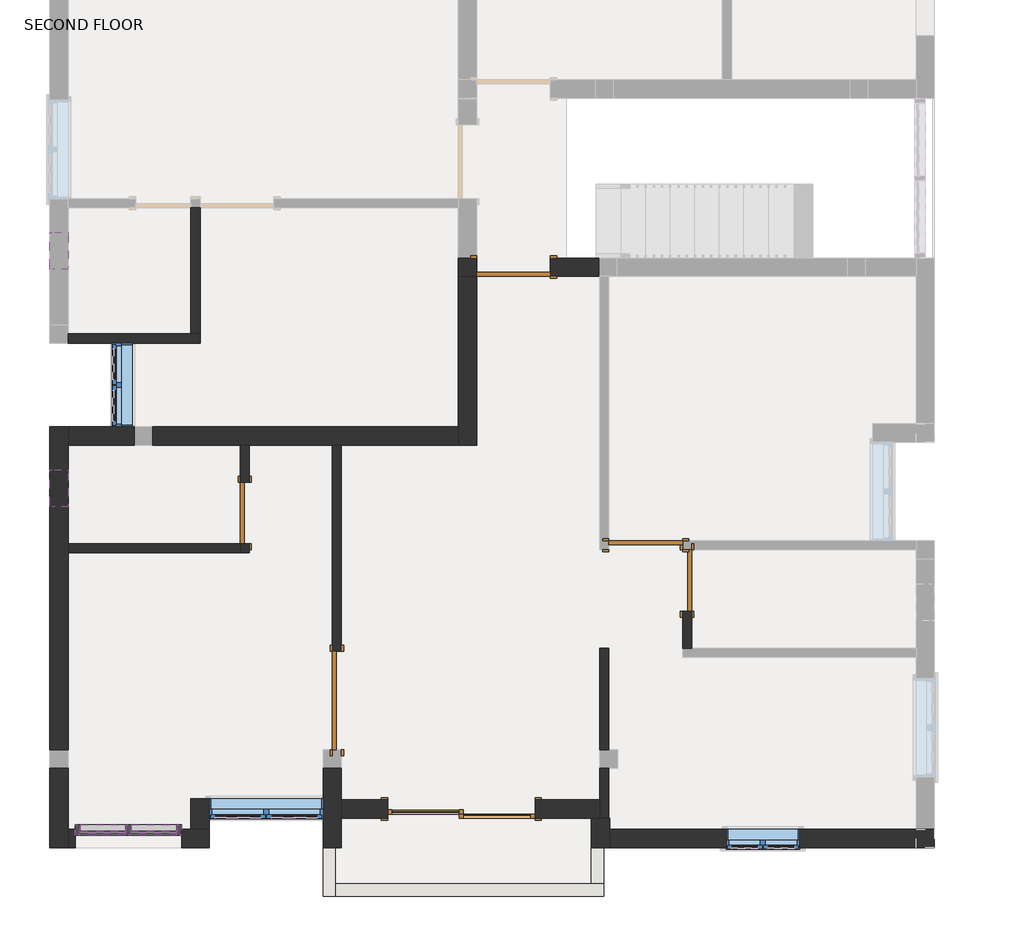
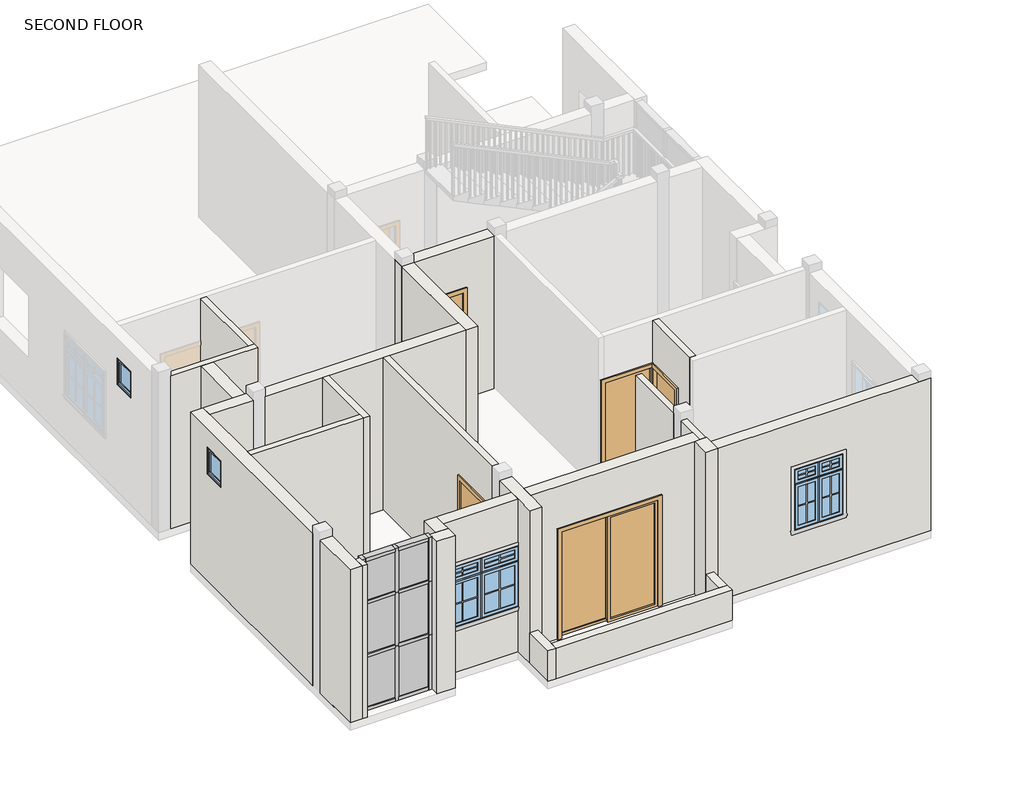
# One storey, part 1 of 6: 25 walls, 17 members, 6 doors, 6 plates, 5 windows.
"""IFC4 building model written with IfcOpenShell, lengths in millimetres."""

from ifc_helpers import new_model, si_unit, frame, origin, place, context, project, spatial, polyline, outline, extrude, faceted_brep, transform, mapped, element, save
from components import door_d4d75d1e, door_78caadf7, single_flush_3_x7_0ca8825f, single_flush_3_x7_305aa2a5, single_flush_4_x7_9343de66, member_6f432376, member_6103f85b, member_e80433b6, member_a715cb85, member_69c8e218, member_c4de40ee, member_049a2e78, member_5cd4c5ac, system_panel_glazed_fbef02e7, system_panel_glazed_b4a8312c, window_abb441dd, window_35f3c129, window_casement_double_awning_double_3_x4_7dc4ce09, window_c5cb33f6

model = new_model("IFC4")

# Units and contexts
model_context = context("Model", 3, world=origin())
ifc_project = project(units=[si_unit("LENGTHUNIT", "METRE", prefix="MILLI")], contexts=[model_context])

# Site, building, storey
site = spatial("IfcSite", under=ifc_project)
building = spatial("IfcBuilding", under=site)
storey = spatial("IfcBuildingStorey", under=building, Name="SECOND FLOOR", Elevation=6400.8)

# Doors
placement = place(None, origin())
door_shape = door_d4d75d1e(model_context)
element("IfcDoor", 1, ObjectType="Door-Double-Sliding : 72\" x 84\"", at=placement, inside=storey, context=model_context, shape_type="MappedRepresentation", body=[
    mapped(door_shape, transform((-1663.0865981, -7209.8212413, 6400.8), x_axis=(-1.0, 0.0, 0.0), y_axis=(0.0, -1.0, 0.0), z_axis=(0.0, 0.0, 1.0))),
])
door_2_shape = door_78caadf7(model_context)
element("IfcDoor", 2, ObjectType="Single-Flush : 2'6\"X7'", at=placement, inside=storey, context=model_context, shape_type="MappedRepresentation", body=[
    mapped(door_2_shape, transform((-4349.1365981, -3666.5212413, 6400.8), x_axis=(0.0, -1.0, 0.0), y_axis=(1.0, 0.0, 0.0), z_axis=(0.0, 0.0, 1.0))),
])
element("IfcDoor", 3, ObjectType="Single-Flush : 2'6\"X7'", at=placement, inside=storey, context=model_context, shape_type="MappedRepresentation", body=[
    mapped(door_2_shape, transform((1137.2634019, -4504.7212413, 6400.8), x_axis=(0.0, 1.0, 0.0), y_axis=(-1.0, 0.0, 0.0), z_axis=(0.0, 0.0, 1.0))),
])
single_flush_3_x7_shape = single_flush_3_x7_0ca8825f(model_context)
element("IfcDoor", 4, ObjectType="Single-Flush : 3'X7'", at=placement, inside=storey, context=model_context, shape_type="MappedRepresentation", body=[
    mapped(single_flush_3_x7_shape, transform((-1015.3865981, -618.5212413, 6400.8), x_axis=(-1.0, 0.0, 0.0), y_axis=(0.0, -1.0, 0.0), z_axis=(0.0, 0.0, 1.0))),
])
single_flush_3_x7_2_shape = single_flush_3_x7_305aa2a5(model_context)
element("IfcDoor", 5, ObjectType="Single-Flush : 3'X7'", at=placement, inside=storey, context=model_context, shape_type="MappedRepresentation", body=[
    mapped(single_flush_3_x7_2_shape, transform((622.9134019, -4066.5712413, 6400.8), x_axis=(-1.0, 0.0, 0.0), y_axis=(0.0, -1.0, 0.0), z_axis=(0.0, 0.0, 1.0))),
])
single_flush_4_x7_shape = single_flush_4_x7_9343de66(model_context)
element("IfcDoor", 6, ObjectType="Single-Flush : 4'X7'", at=placement, inside=storey, context=model_context, shape_type="MappedRepresentation", body=[
    mapped(single_flush_4_x7_shape, transform((-3206.1365981, -5990.6212413, 6400.8), x_axis=(0.0, -1.0, 0.0), y_axis=(1.0, 0.0, 0.0), z_axis=(0.0, 0.0, 1.0))),
])

# Members
member_shape = member_6f432376(model_context)
element("IfcMember", 7, ObjectType="Rectangular Mullion : 2.5\" x 5\" rectangular", at=placement, inside=storey, context=model_context, shape_type="MappedRepresentation", body=[
    mapped(member_shape, transform((-5193.6865981, -7597.1712413, 9448.8), x_axis=(0.0, 0.0, 1.0), y_axis=(0.0, -1.0, 0.0), z_axis=(1.0, 0.0, 0.0))),
])
element("IfcMember", 8, ObjectType="Rectangular Mullion : 2.5\" x 5\" rectangular", at=placement, inside=storey, context=model_context, shape_type="MappedRepresentation", body=[
    mapped(member_shape, transform((-5822.3365981, -7597.1712413, 9448.8), x_axis=(0.0, 0.0, 1.0), y_axis=(0.0, -1.0, 0.0), z_axis=(1.0, 0.0, 0.0))),
])
element("IfcMember", 9, ObjectType="Rectangular Mullion : 2.5\" x 5\" rectangular", at=placement, inside=storey, context=model_context, shape_type="MappedRepresentation", body=[
    mapped(member_shape, transform((-6387.4865981, -7597.1712413, 6400.8), x_axis=(0.0, 0.0, -1.0), y_axis=(0.0, -1.0, 0.0), z_axis=(-1.0, 0.0, 0.0))),
])
element("IfcMember", 10, ObjectType="Rectangular Mullion : 2.5\" x 5\" rectangular", at=placement, inside=storey, context=model_context, shape_type="MappedRepresentation", body=[
    mapped(member_shape, transform((-5758.8365981, -7597.1712413, 6400.8), x_axis=(0.0, 0.0, -1.0), y_axis=(0.0, -1.0, 0.0), z_axis=(-1.0, 0.0, 0.0))),
])
member_2_shape = member_6103f85b(model_context)
element("IfcMember", 11, ObjectType="Rectangular Mullion : 2.5\" x 5\" rectangular", at=placement, inside=storey, context=model_context, shape_type="MappedRepresentation", body=[
    mapped(member_2_shape, transform((-5822.3365981, -7597.1712413, 7499.35), x_axis=(0.0, 0.0, 1.0), y_axis=(0.0, -1.0, 0.0), z_axis=(1.0, 0.0, 0.0))),
])
element("IfcMember", 12, ObjectType="Rectangular Mullion : 2.5\" x 5\" rectangular", at=placement, inside=storey, context=model_context, shape_type="MappedRepresentation", body=[
    mapped(member_2_shape, transform((-5822.3365981, -7597.1712413, 8566.15), x_axis=(0.0, 0.0, 1.0), y_axis=(0.0, -1.0, 0.0), z_axis=(1.0, 0.0, 0.0))),
])
element("IfcMember", 13, ObjectType="Rectangular Mullion : 2.5\" x 5\" rectangular", at=placement, inside=storey, context=model_context, shape_type="MappedRepresentation", body=[
    mapped(member_2_shape, transform((-5193.6865981, -7597.1712413, 7499.35), x_axis=(0.0, 0.0, 1.0), y_axis=(0.0, -1.0, 0.0), z_axis=(1.0, 0.0, 0.0))),
])
element("IfcMember", 14, ObjectType="Rectangular Mullion : 2.5\" x 5\" rectangular", at=placement, inside=storey, context=model_context, shape_type="MappedRepresentation", body=[
    mapped(member_2_shape, transform((-5193.6865981, -7597.1712413, 8566.15), x_axis=(0.0, 0.0, 1.0), y_axis=(0.0, -1.0, 0.0), z_axis=(1.0, 0.0, 0.0))),
])
member_3_shape = member_e80433b6(model_context)
element("IfcMember", 15, ObjectType="Rectangular Mullion : 2.5\" x 5\" rectangular", at=placement, inside=storey, context=model_context, shape_type="MappedRepresentation", body=[
    mapped(member_3_shape, transform((-5790.5865981, -7597.1712413, 6400.8), x_axis=(1.0, 0.0, 0.0), y_axis=(0.0, -1.0, 0.0), z_axis=(0.0, 0.0, -1.0))),
])
member_4_shape = member_a715cb85(model_context)
element("IfcMember", 16, ObjectType="Rectangular Mullion : 2.5\" x 5\" rectangular", at=placement, inside=storey, context=model_context, shape_type="MappedRepresentation", body=[
    mapped(member_4_shape, transform((-5790.5865981, -7597.1712413, 7499.35), x_axis=(1.0, 0.0, 0.0), y_axis=(0.0, -1.0, 0.0), z_axis=(0.0, 0.0, -1.0))),
])
member_5_shape = member_69c8e218(model_context)
element("IfcMember", 17, ObjectType="Rectangular Mullion : 2.5\" x 5\" rectangular", at=placement, inside=storey, context=model_context, shape_type="MappedRepresentation", body=[
    mapped(member_5_shape, transform((-5130.1865981, -7597.1712413, 6400.8), x_axis=(1.0, 0.0, 0.0), y_axis=(0.0, -1.0, 0.0), z_axis=(0.0, 0.0, -1.0))),
])
member_6_shape = member_c4de40ee(model_context)
element("IfcMember", 18, ObjectType="Rectangular Mullion : 2.5\" x 5\" rectangular", at=placement, inside=storey, context=model_context, shape_type="MappedRepresentation", body=[
    mapped(member_6_shape, transform((-5130.1865981, -7597.1712413, 7499.35), x_axis=(1.0, 0.0, 0.0), y_axis=(0.0, -1.0, 0.0), z_axis=(0.0, 0.0, -1.0))),
])
element("IfcMember", 19, ObjectType="Rectangular Mullion : 2.5\" x 5\" rectangular", at=placement, inside=storey, context=model_context, shape_type="MappedRepresentation", body=[
    mapped(member_5_shape, transform((-6450.9865981, -7597.1712413, 7499.35), x_axis=(-1.0, 0.0, 0.0), y_axis=(0.0, -1.0, 0.0), z_axis=(0.0, 0.0, 1.0))),
])
element("IfcMember", 20, ObjectType="Rectangular Mullion : 2.5\" x 5\" rectangular", at=placement, inside=storey, context=model_context, shape_type="MappedRepresentation", body=[
    mapped(member_6_shape, transform((-6450.9865981, -7597.1712413, 8566.15), x_axis=(-1.0, 0.0, 0.0), y_axis=(0.0, -1.0, 0.0), z_axis=(0.0, 0.0, 1.0))),
])
member_7_shape = member_049a2e78(model_context)
element("IfcMember", 21, ObjectType="Rectangular Mullion : 2.5\" x 5\" rectangular", at=placement, inside=storey, context=model_context, shape_type="MappedRepresentation", body=[
    mapped(member_7_shape, transform((-5790.5865981, -7597.1712413, 8566.15), x_axis=(1.0, 0.0, 0.0), y_axis=(0.0, -1.0, 0.0), z_axis=(0.0, 0.0, -1.0))),
])
member_8_shape = member_5cd4c5ac(model_context)
element("IfcMember", 22, ObjectType="Rectangular Mullion : 2.5\" x 5\" rectangular", at=placement, inside=storey, context=model_context, shape_type="MappedRepresentation", body=[
    mapped(member_8_shape, transform((-5130.1865981, -7597.1712413, 8566.15), x_axis=(1.0, 0.0, 0.0), y_axis=(0.0, -1.0, 0.0), z_axis=(0.0, 0.0, -1.0))),
])
element("IfcMember", 23, ObjectType="Rectangular Mullion : 2.5\" x 5\" rectangular", at=placement, inside=storey, context=model_context, shape_type="MappedRepresentation", body=[
    mapped(member_8_shape, transform((-6450.9865981, -7597.1712413, 9448.8), x_axis=(-1.0, 0.0, 0.0), y_axis=(0.0, -1.0, 0.0), z_axis=(0.0, 0.0, 1.0))),
])

# Plates
system_panel_glazed_shape = system_panel_glazed_fbef02e7(model_context)
element("IfcPlate", 24, ObjectType="System Panel : Glazed", at=placement, inside=storey, context=model_context, shape_type="MappedRepresentation", body=[
    mapped(system_panel_glazed_shape, transform((-6104.9115981, -7597.1712413, 6464.3), x_axis=(1.0, 0.0, 0.0), y_axis=(0.0, 1.0, 0.0), z_axis=(0.0, 0.0, 1.0))),
])
element("IfcPlate", 25, ObjectType="System Panel : Glazed", at=placement, inside=storey, context=model_context, shape_type="MappedRepresentation", body=[
    mapped(system_panel_glazed_shape, transform((-6104.9115981, -7597.1712413, 7531.1), x_axis=(1.0, 0.0, 0.0), y_axis=(0.0, 1.0, 0.0), z_axis=(0.0, 0.0, 1.0))),
])
element("IfcPlate", 26, ObjectType="System Panel : Glazed", at=placement, inside=storey, context=model_context, shape_type="MappedRepresentation", body=[
    mapped(system_panel_glazed_shape, transform((-5476.2615981, -7597.1712413, 6464.3), x_axis=(1.0, 0.0, 0.0), y_axis=(0.0, 1.0, 0.0), z_axis=(0.0, 0.0, 1.0))),
])
element("IfcPlate", 27, ObjectType="System Panel : Glazed", at=placement, inside=storey, context=model_context, shape_type="MappedRepresentation", body=[
    mapped(system_panel_glazed_shape, transform((-5476.2615981, -7597.1712413, 7531.1), x_axis=(1.0, 0.0, 0.0), y_axis=(0.0, 1.0, 0.0), z_axis=(0.0, 0.0, 1.0))),
])
system_panel_glazed_2_shape = system_panel_glazed_b4a8312c(model_context)
element("IfcPlate", 28, ObjectType="System Panel : Glazed", at=placement, inside=storey, context=model_context, shape_type="MappedRepresentation", body=[
    mapped(system_panel_glazed_2_shape, transform((-6104.9115981, -7597.1712413, 8597.9), x_axis=(1.0, 0.0, 0.0), y_axis=(0.0, 1.0, 0.0), z_axis=(0.0, 0.0, 1.0))),
])
element("IfcPlate", 29, ObjectType="System Panel : Glazed", at=placement, inside=storey, context=model_context, shape_type="MappedRepresentation", body=[
    mapped(system_panel_glazed_2_shape, transform((-5476.2615981, -7597.1712413, 8597.9), x_axis=(1.0, 0.0, 0.0), y_axis=(0.0, 1.0, 0.0), z_axis=(0.0, 0.0, 1.0))),
])

# Walls
element("IfcWall", 30, ObjectType="4.5\"", at=placement, inside=storey, context=model_context, shape_type="Brep", body=[
    faceted_brep([(-6539.8865981, -1558.3212413, 6400.8), (-5974.2886947, -1558.3212413, 6400.8), (-5745.6886947, -1558.3212413, 6400.8), (-4901.5865981, -1558.3212413, 6400.8), (-4901.5865981, -1558.3212413, 9448.8), (-5745.6886947, -1558.3212413, 9448.8), (-5974.2886947, -1558.3212413, 9448.8), (-6539.8865981, -1558.3212413, 9448.8), (-6539.8865981, -1444.0212413, 6400.8), (-6539.8865981, -1444.0212413, 9448.8), (-5015.8865981, -1444.0212413, 9448.8), (-4901.5865981, -1444.0212413, 9448.8), (-4901.5865981, -1444.0212413, 6400.8), (-5015.8865981, -1444.0212413, 6400.8)], [[[0, 1, 2, 3, 4, 5, 6, 7]], [[8, 9, 10, 11, 12, 13]], [[3, 2, 1, 0, 8, 13, 12]], [[7, 6, 5, 4, 11, 10, 9]], [[0, 7, 9, 8]], [[4, 3, 12, 11]]]),
])
element("IfcWall", 31, ObjectType="4.5\"", at=placement, inside=storey, context=model_context, shape_type="SweptSolid", body=[
    extrude(outline(polyline([(-4901.5865981, 118.0787587), (-4901.5865981, -1444.0212413), (-5015.8865981, -1444.0212413), (-5015.8865981, 118.0787587), (-4901.5865981, 118.0787587)])), frame((0.0, 0.0, 6400.8), z_axis=(0.0, 0.0, 1.0), x_axis=(1.0, 0.0, 0.0)), (0.0, 0.0, 1.0), 3048.0),
])
element("IfcWall", 32, ObjectType="4.5\"", at=placement, inside=storey, context=model_context, shape_type="Brep", body=[
    faceted_brep([(-4406.2865981, -4047.5212413, 8534.4), (-4406.2865981, -4047.5212413, 6400.8), (-4406.2865981, -4161.8212413, 6400.8), (-4406.2865981, -4161.8212413, 9448.8), (-4406.2865981, -4047.5212413, 9448.8), (-4406.2865981, -2828.3212413, 9448.8), (-4406.2865981, -2828.3212413, 6400.8), (-4406.2865981, -3285.5212413, 6400.8), (-4406.2865981, -3285.5212413, 8534.4), (-4291.9865981, -4161.8212413, 6400.8), (-4291.9865981, -4047.5212413, 6400.8), (-4291.9865981, -4047.5212413, 8534.4), (-4291.9865981, -3285.5212413, 8534.4), (-4291.9865981, -3285.5212413, 6400.8), (-4291.9865981, -2828.3212413, 6400.8), (-4291.9865981, -2828.3212413, 9448.8), (-4291.9865981, -4161.8212413, 9448.8)], [[[0, 1, 2, 3, 4, 5, 6, 7, 8]], [[9, 10, 11, 12, 13, 14, 15, 16]], [[7, 6, 14, 13]], [[2, 1, 10, 9]], [[5, 4, 3, 16, 15]], [[6, 5, 15, 14]], [[3, 2, 9, 16]], [[11, 10, 1, 0]], [[12, 11, 0, 8]], [[13, 12, 8, 7]]]),
])
element("IfcWall", 33, ObjectType="4.5\"", at=placement, inside=storey, context=model_context, shape_type="SweptSolid", body=[
    extrude(outline(polyline([(-6539.8865981, -4047.5212413), (-4406.2865981, -4047.5212413), (-4406.2865981, -4161.8212413), (-6539.8865981, -4161.8212413), (-6539.8865981, -4047.5212413)])), frame((0.0, 0.0, 6400.8), z_axis=(0.0, 0.0, 1.0), x_axis=(1.0, 0.0, 0.0)), (0.0, 0.0, 1.0), 3048.0),
])
element("IfcWall", 34, ObjectType="4.5\"", at=placement, inside=storey, context=model_context, shape_type="SweptSolid", body=[
    extrude(outline(polyline([(-6600.2212413, 9448.8), (-2828.3212413, 9448.8), (-2828.3212413, 6400.8), (-5381.0212413, 6400.8), (-5381.0212413, 8534.4), (-6600.2212413, 8534.4), (-6600.2212413, 9448.8)])), frame((-3263.2865981, 0.0, 0.0), z_axis=(1.0, 0.0, 0.0), x_axis=(0.0, 1.0, 0.0)), (0.0, 0.0, 1.0), 114.3),
])
element("IfcWall", 35, ObjectType="4.5\"", at=placement, inside=storey, context=model_context, shape_type="SweptSolid", body=[
    extrude(outline(polyline([(-5342.9212413, 9448.8), (-4123.7212413, 9448.8), (-4123.7212413, 8534.4), (-4885.7212413, 8534.4), (-4885.7212413, 6400.8), (-5342.9212413, 6400.8), (-5342.9212413, 9448.8)])), frame((1080.1134019, 0.0, 0.0), z_axis=(1.0, 0.0, 0.0), x_axis=(0.0, 1.0, 0.0)), (0.0, 0.0, 1.0), 114.3),
])
element("IfcWall", 36, ObjectType="4.5\"", at=placement, inside=storey, context=model_context, shape_type="SweptSolid", body=[
    extrude(outline(polyline([(51.4134019, -6601.1424416), (51.4134019, -5342.9212413), (165.7134019, -5342.9212413), (165.7134019, -6601.1424416), (51.4134019, -6601.1424416)])), frame((0.0, 0.0, 6400.8), z_axis=(0.0, 0.0, 1.0), x_axis=(1.0, 0.0, 0.0)), (0.0, 0.0, 1.0), 3048.0),
])
element("IfcWall", 37, ObjectType="4.5\"", at=placement, inside=storey, context=model_context, shape_type="Brep", body=[
    faceted_brep([(51.4134019, -6829.7424416, 6400.8), (51.4134019, -7222.5212413, 6400.8), (51.4134019, -7451.1212413, 6400.8), (51.4134019, -7451.1212413, 9448.8), (51.4134019, -7222.5212413, 9448.8), (51.4134019, -6829.7424416, 9448.8), (165.7134019, -6829.7424416, 6400.8), (165.7134019, -6829.7424416, 9448.8), (165.7134019, -7451.1212413, 9448.8), (165.7134019, -7451.1212413, 6400.8)], [[[0, 1, 2, 3, 4, 5]], [[6, 7, 8, 9]], [[2, 1, 0, 6, 9]], [[5, 4, 3, 8, 7]], [[0, 5, 7, 6]], [[3, 2, 9, 8]]]),
])
element("IfcWall", 38, ObjectType="6\"", at=placement, inside=storey, context=model_context, shape_type="Brep", body=[
    faceted_brep([(-3377.5865981, -7819.4212413, 6400.8), (-3377.5865981, -8416.3212413, 6400.8), (-3377.5865981, -8416.3212413, 7010.4), (-3377.5865981, -7819.4212413, 7010.4), (-3225.1865981, -7819.4212413, 6400.8), (-3225.1865981, -7819.4212413, 7010.4), (-3225.1865981, -8263.9212413, 7010.4), (-3225.1865981, -8416.3212413, 7010.4), (-3225.1865981, -8416.3212413, 6400.8), (-3225.1865981, -8263.9212413, 6400.8)], [[[0, 1, 2, 3]], [[4, 5, 6, 7, 8, 9]], [[1, 0, 4, 9, 8]], [[3, 2, 7, 6, 5]], [[0, 3, 5, 4]], [[2, 1, 8, 7]]]),
])
element("IfcWall", 39, ObjectType="6\"", at=placement, inside=storey, context=model_context, shape_type="Brep", body=[
    faceted_brep([(-3225.1865981, -8416.3212413, 6400.8), (102.2134019, -8416.3212413, 6400.8), (102.2134019, -8416.3212413, 7010.4), (-3225.1865981, -8416.3212413, 7010.4), (-3225.1865981, -8263.9212413, 6400.8), (-3225.1865981, -8263.9212413, 7010.4), (-50.1865981, -8263.9212413, 7010.4), (102.2134019, -8263.9212413, 7010.4), (102.2134019, -8263.9212413, 6400.8), (-50.1865981, -8263.9212413, 6400.8)], [[[0, 1, 2, 3]], [[4, 5, 6, 7, 8, 9]], [[1, 0, 4, 9, 8]], [[3, 2, 7, 6, 5]], [[0, 3, 5, 4]], [[2, 1, 8, 7]]]),
])
element("IfcWall", 40, ObjectType="6\"", at=placement, inside=storey, context=model_context, shape_type="SweptSolid", body=[
    extrude(outline(polyline([(102.2134019, -7819.4212413), (102.2134019, -8263.9212413), (-50.1865981, -8263.9212413), (-50.1865981, -7819.4212413), (102.2134019, -7819.4212413)])), frame((0.0, 0.0, 6400.8), z_axis=(0.0, 0.0, 1.0), x_axis=(1.0, 0.0, 0.0)), (0.0, 0.0, 1.0), 609.6),
])
element("IfcWall", 41, ObjectType="9\"", at=placement, inside=storey, context=model_context, shape_type="Brep", body=[
    faceted_brep([(-6768.4865981, -2599.7212413, 6400.8), (-6768.4865981, -6601.1424416, 6400.8), (-6768.4865981, -6601.1424416, 9448.8), (-6768.4865981, -2599.7212413, 9448.8), (-6768.4865981, -3133.1212413, 9067.8), (-6768.4865981, -3590.3212413, 9067.8), (-6768.4865981, -3590.3212413, 8534.4), (-6768.4865981, -3133.1212413, 8534.4), (-6539.8865981, -2599.7212413, 6400.8), (-6539.8865981, -2599.7212413, 9448.8), (-6539.8865981, -2828.3212413, 9448.8), (-6539.8865981, -4047.5212413, 9448.8), (-6539.8865981, -4161.8212413, 9448.8), (-6539.8865981, -6601.1424416, 9448.8), (-6539.8865981, -6601.1424416, 6400.8), (-6539.8865981, -4161.8212413, 6400.8), (-6539.8865981, -4047.5212413, 6400.8), (-6539.8865981, -2828.3212413, 6400.8), (-6539.8865981, -3133.1212413, 9067.8), (-6539.8865981, -3133.1212413, 8534.4), (-6539.8865981, -3590.3212413, 8534.4), (-6539.8865981, -3590.3212413, 9067.8)], [[[0, 1, 2, 3], [4, 5, 6, 7]], [[8, 9, 10, 11, 12, 13, 14, 15, 16, 17], [18, 19, 20, 21]], [[1, 0, 8, 17, 16, 15, 14]], [[2, 1, 14, 13]], [[3, 2, 13, 12, 11, 10, 9]], [[0, 3, 9, 8]], [[19, 18, 4, 7]], [[20, 19, 7, 6]], [[21, 20, 6, 5]], [[18, 21, 5, 4]]]),
])
element("IfcWall", 42, ObjectType="9\"", at=placement, inside=storey, context=model_context, shape_type="Brep", body=[
    faceted_brep([(-6768.4865981, -6829.7424416, 6400.8), (-6768.4865981, -7819.4212413, 6400.8), (-6768.4865981, -7819.4212413, 9448.8), (-6768.4865981, -6829.7424416, 9448.8), (-6539.8865981, -6829.7424416, 6400.8), (-6539.8865981, -6829.7424416, 9448.8), (-6539.8865981, -7590.8212413, 9448.8), (-6539.8865981, -7819.4212413, 9448.8), (-6539.8865981, -7819.4212413, 6400.8), (-6539.8865981, -7590.8212413, 6400.8)], [[[0, 1, 2, 3]], [[4, 5, 6, 7, 8, 9]], [[1, 0, 4, 9, 8]], [[3, 2, 7, 6, 5]], [[0, 3, 5, 4]], [[2, 1, 8, 7]]]),
])
element("IfcWall", 43, ObjectType="9\"", at=placement, inside=storey, context=model_context, shape_type="Brep", body=[
    faceted_brep([(-6539.8865981, -7819.4212413, 9448.8), (-6539.8865981, -7819.4212413, 6400.8), (-6450.9865981, -7819.4212413, 6400.8), (-6450.9865981, -7819.4212413, 9448.8), (-6539.8865981, -7590.8212413, 6400.8), (-6539.8865981, -7590.8212413, 9448.8), (-6450.9865981, -7590.8212413, 9448.8), (-6450.9865981, -7590.8212413, 6400.8)], [[[0, 1, 2, 3]], [[4, 5, 6, 7]], [[1, 4, 7, 2]], [[5, 0, 3, 6]], [[1, 0, 5, 4]], [[3, 2, 7, 6]]]),
    faceted_brep([(-4787.2865981, -7819.4212413, 6400.8), (-4787.2865981, -7819.4212413, 9448.8), (-5130.1865981, -7819.4212413, 9448.8), (-5130.1865981, -7819.4212413, 6400.8), (-4787.2865981, -7590.8212413, 9448.8), (-4787.2865981, -7590.8212413, 6400.8), (-5015.8865981, -7590.8212413, 6400.8), (-5130.1865981, -7590.8212413, 6400.8), (-5130.1865981, -7590.8212413, 9448.8), (-5015.8865981, -7590.8212413, 9448.8)], [[[0, 1, 2, 3]], [[4, 5, 6, 7, 8, 9]], [[5, 0, 3, 7, 6]], [[1, 4, 9, 8, 2]], [[1, 0, 5, 4]], [[3, 2, 8, 7]]]),
])
element("IfcWall", 44, ObjectType="9\"", at=placement, inside=storey, context=model_context, shape_type="Brep", body=[
    faceted_brep([(-4787.2865981, -7590.8212413, 6400.8), (-4787.2865981, -7438.4212413, 6400.8), (-4787.2865981, -7209.8212413, 6400.8), (-4787.2865981, -7209.8212413, 7315.2), (-4787.2865981, -7209.8212413, 8534.4), (-4787.2865981, -7209.8212413, 9448.8), (-4787.2865981, -7438.4212413, 9448.8), (-4787.2865981, -7590.8212413, 9448.8), (-5015.8865981, -7590.8212413, 6400.8), (-5015.8865981, -7590.8212413, 9448.8), (-5015.8865981, -7209.8212413, 9448.8), (-5015.8865981, -7209.8212413, 6400.8)], [[[0, 1, 2, 3, 4, 5, 6, 7]], [[8, 9, 10, 11]], [[2, 1, 0, 8, 11]], [[7, 6, 5, 10, 9]], [[0, 7, 9, 8]], [[5, 4, 3, 2, 11, 10]]]),
])
element("IfcWall", 45, ObjectType="9\"", at=placement, inside=storey, context=model_context, shape_type="SweptSolid", body=[
    extrude(outline(polyline([(-3377.5865981, -7438.4212413), (-4787.2865981, -7438.4212413), (-4787.2865981, -7209.8212413), (-3377.5865981, -7209.8212413), (-3377.5865981, -7438.4212413)])), frame((0.0, 0.0, 6400.8), z_axis=(0.0, 0.0, 1.0), x_axis=(1.0, 0.0, 0.0)), (0.0, 0.0, 1.0), 914.4),
    extrude(outline(polyline([(-3377.5865981, -7438.4212413), (-4787.2865981, -7438.4212413), (-4787.2865981, -7209.8212413), (-3377.5865981, -7209.8212413), (-3377.5865981, -7438.4212413)])), frame((0.0, 0.0, 8534.4), z_axis=(0.0, 0.0, 1.0), x_axis=(1.0, 0.0, 0.0)), (0.0, 0.0, 1.0), 914.4),
])
element("IfcWall", 46, ObjectType="9\"", at=placement, inside=storey, context=model_context, shape_type="Brep", body=[
    faceted_brep([(-3377.5865981, -6828.8212413, 6400.8), (-3377.5865981, -7209.8212413, 6400.8), (-3377.5865981, -7438.4212413, 6400.8), (-3377.5865981, -7819.4212413, 6400.8), (-3377.5865981, -7819.4212413, 7010.4), (-3377.5865981, -7819.4212413, 9448.8), (-3377.5865981, -7438.4212413, 9448.8), (-3377.5865981, -7209.8212413, 9448.8), (-3377.5865981, -6828.8212413, 9448.8), (-3148.9865981, -6828.8212413, 6400.8), (-3148.9865981, -6828.8212413, 9448.8), (-3148.9865981, -7222.5212413, 9448.8), (-3148.9865981, -7451.1212413, 9448.8), (-3148.9865981, -7819.4212413, 9448.8), (-3148.9865981, -7819.4212413, 6400.8), (-3148.9865981, -7451.1212413, 6400.8), (-3148.9865981, -7222.5212413, 6400.8), (-3225.1865981, -7819.4212413, 6400.8)], [[[0, 1, 2, 3, 4, 5, 6, 7, 8]], [[9, 10, 11, 12, 13, 14, 15, 16]], [[3, 2, 1, 0, 9, 16, 15, 14, 17]], [[5, 4, 3, 17, 14, 13]], [[8, 7, 6, 5, 13, 12, 11, 10]], [[0, 8, 10, 9]]]),
])
element("IfcWall", 47, ObjectType="9\"", at=placement, inside=storey, context=model_context, shape_type="Brep", body=[
    faceted_brep([(-2577.4865981, -7222.5212413, 8534.4), (-2577.4865981, -7222.5212413, 6400.8), (-3148.9865981, -7222.5212413, 6400.8), (-3148.9865981, -7222.5212413, 9448.8), (51.4134019, -7222.5212413, 9448.8), (51.4134019, -7222.5212413, 6400.8), (-748.6865981, -7222.5212413, 6400.8), (-748.6865981, -7222.5212413, 8534.4), (-3148.9865981, -7451.1212413, 6400.8), (-2577.4865981, -7451.1212413, 6400.8), (-2577.4865981, -7451.1212413, 8534.4), (-748.6865981, -7451.1212413, 8534.4), (-748.6865981, -7451.1212413, 6400.8), (-50.1865981, -7451.1212413, 6400.8), (51.4134019, -7451.1212413, 6400.8), (51.4134019, -7451.1212413, 9448.8), (-50.1865981, -7451.1212413, 9448.8), (-3148.9865981, -7451.1212413, 9448.8)], [[[0, 1, 2, 3, 4, 5, 6, 7]], [[8, 9, 10, 11, 12, 13, 14, 15, 16, 17]], [[6, 5, 14, 13, 12]], [[2, 1, 9, 8]], [[4, 3, 17, 16, 15]], [[3, 2, 8, 17]], [[5, 4, 15, 14]], [[12, 11, 7, 6]], [[10, 9, 1, 0]], [[11, 10, 0, 7]]]),
])
element("IfcWall", 48, ObjectType="9\"", at=placement, inside=storey, context=model_context, shape_type="Brep", body=[
    faceted_brep([(-50.1865981, -7451.1212413, 6400.8), (-50.1865981, -7819.4212413, 6400.8), (-50.1865981, -7819.4212413, 7010.4), (-50.1865981, -7819.4212413, 9448.8), (-50.1865981, -7451.1212413, 9448.8), (178.4134019, -7451.1212413, 6400.8), (178.4134019, -7451.1212413, 9448.8), (178.4134019, -7590.8212413, 9448.8), (178.4134019, -7819.4212413, 9448.8), (178.4134019, -7819.4212413, 6400.8), (178.4134019, -7590.8212413, 6400.8), (51.4134019, -7451.1212413, 6400.8), (165.7134019, -7451.1212413, 6400.8), (102.2134019, -7819.4212413, 6400.8), (165.7134019, -7451.1212413, 9448.8), (51.4134019, -7451.1212413, 9448.8)], [[[0, 1, 2, 3, 4]], [[5, 6, 7, 8, 9, 10]], [[1, 0, 11, 12, 5, 10, 9, 13]], [[4, 3, 8, 7, 6, 14, 15]], [[0, 4, 15, 14, 6, 5, 12, 11]], [[1, 13, 9, 8, 3, 2]]]),
])
element("IfcWall", 49, ObjectType="9\"", at=placement, inside=storey, context=model_context, shape_type="Brep", body=[
    faceted_brep([(178.4134019, -7819.4212413, 9448.8), (178.4134019, -7819.4212413, 6400.8), (4204.3134019, -7819.4212413, 6400.8), (4204.3134019, -7819.4212413, 9448.8), (3975.7134019, -7819.4212413, 9448.8), (1619.8634019, -7819.4212413, 8534.4), (2534.2634019, -7819.4212413, 8534.4), (2534.2634019, -7819.4212413, 7315.2), (1619.8634019, -7819.4212413, 7315.2), (178.4134019, -7590.8212413, 6400.8), (178.4134019, -7590.8212413, 9448.8), (3975.7134019, -7590.8212413, 9448.8), (4204.3134019, -7590.8212413, 9448.8), (4204.3134019, -7590.8212413, 6400.8), (3975.7134019, -7590.8212413, 6400.8), (1619.8634019, -7590.8212413, 8534.4), (1619.8634019, -7590.8212413, 7315.2), (2534.2634019, -7590.8212413, 7315.2), (2534.2634019, -7590.8212413, 8534.4)], [[[0, 1, 2, 3, 4], [5, 6, 7, 8]], [[9, 10, 11, 12, 13, 14], [15, 16, 17, 18]], [[2, 1, 9, 14, 13]], [[0, 4, 3, 12, 11, 10]], [[3, 2, 13, 12]], [[0, 10, 9, 1]], [[16, 15, 5, 8]], [[17, 16, 8, 7]], [[18, 17, 7, 6]], [[15, 18, 6, 5]]]),
])
element("IfcWall", 50, ObjectType="9\"", at=placement, inside=storey, context=model_context, shape_type="Brep", body=[
    faceted_brep([(-1472.5865981, -504.2212413, 8534.4), (-1472.5865981, -504.2212413, 6400.8), (-1701.1865981, -504.2212413, 6400.8), (-1701.1865981, -504.2212413, 9448.8), (-1472.5865981, -504.2212413, 9448.8), (41.1035962, -504.2212413, 9448.8), (41.1035962, -504.2212413, 6400.8), (-558.1865981, -504.2212413, 6400.8), (-558.1865981, -504.2212413, 8534.4), (-1701.1865981, -732.8212413, 6400.8), (-1472.5865981, -732.8212413, 6400.8), (-1472.5865981, -732.8212413, 8534.4), (-558.1865981, -732.8212413, 8534.4), (-558.1865981, -732.8212413, 6400.8), (41.1035962, -732.8212413, 6400.8), (41.1035962, -732.8212413, 9448.8), (-1472.5865981, -732.8212413, 9448.8), (-1701.1865981, -732.8212413, 9448.8), (-1701.1865981, -505.1424416, 9448.8)], [[[0, 1, 2, 3, 4, 5, 6, 7, 8]], [[9, 10, 11, 12, 13, 14, 15, 16, 17]], [[7, 6, 14, 13]], [[2, 1, 10, 9]], [[5, 4, 3, 18, 17, 16, 15]], [[6, 5, 15, 14]], [[3, 2, 9, 17, 18]], [[11, 10, 1, 0]], [[12, 11, 0, 8]], [[13, 12, 8, 7]]]),
])
element("IfcWall", 51, ObjectType="9\"", at=placement, inside=storey, context=model_context, shape_type="Brep", body=[
    faceted_brep([(-1701.1865981, -733.7424416, 6400.8), (-1701.1865981, -2599.7212413, 6400.8), (-1701.1865981, -2828.3212413, 6400.8), (-1701.1865981, -2828.3212413, 9448.8), (-1701.1865981, -2599.7212413, 9448.8), (-1701.1865981, -733.7424416, 9448.8), (-1472.5865981, -733.7424416, 6400.8), (-1472.5865981, -733.7424416, 9448.8), (-1472.5865981, -2828.3212413, 9448.8), (-1472.5865981, -2828.3212413, 6400.8)], [[[0, 1, 2, 3, 4, 5]], [[6, 7, 8, 9]], [[2, 1, 0, 6, 9]], [[5, 4, 3, 8, 7]], [[0, 5, 7, 6]], [[3, 2, 9, 8]]]),
])
element("IfcWall", 52, ObjectType="9\"", at=placement, inside=storey, context=model_context, shape_type="Brep", body=[
    faceted_brep([(-1701.1865981, -2599.7212413, 6400.8), (-5488.7582398, -2599.7212413, 6400.8), (-5488.7582398, -2599.7212413, 9448.8), (-1701.1865981, -2599.7212413, 9448.8), (-1701.1865981, -2828.3212413, 6400.8), (-1701.1865981, -2828.3212413, 9448.8), (-3148.9865981, -2828.3212413, 9448.8), (-3263.2865981, -2828.3212413, 9448.8), (-4291.9865981, -2828.3212413, 9448.8), (-4406.2865981, -2828.3212413, 9448.8), (-5488.7582398, -2828.3212413, 9448.8), (-5488.7582398, -2828.3212413, 6400.8), (-4406.2865981, -2828.3212413, 6400.8), (-4291.9865981, -2828.3212413, 6400.8), (-3263.2865981, -2828.3212413, 6400.8), (-3148.9865981, -2828.3212413, 6400.8)], [[[0, 1, 2, 3]], [[4, 5, 6, 7, 8, 9, 10, 11, 12, 13, 14, 15]], [[1, 0, 4, 15, 14, 13, 12, 11]], [[2, 1, 11, 10]], [[3, 2, 10, 9, 8, 7, 6, 5]], [[0, 3, 5, 4]]]),
])
element("IfcWall", 53, ObjectType="9\"", at=placement, inside=storey, context=model_context, shape_type="Brep", body=[
    faceted_brep([(-5717.3582398, -2599.7212413, 6400.8), (-5745.6886947, -2599.7212413, 6400.8), (-5974.2886947, -2599.7212413, 6400.8), (-6539.8865981, -2599.7212413, 6400.8), (-6539.8865981, -2599.7212413, 9448.8), (-5974.2886947, -2599.7212413, 9448.8), (-5745.6886947, -2599.7212413, 9448.8), (-5717.3582398, -2599.7212413, 9448.8), (-5717.3582398, -2828.3212413, 6400.8), (-5717.3582398, -2828.3212413, 9448.8), (-6539.8865981, -2828.3212413, 9448.8), (-6539.8865981, -2828.3212413, 6400.8)], [[[0, 1, 2, 3, 4, 5, 6, 7]], [[8, 9, 10, 11]], [[3, 2, 1, 0, 8, 11]], [[7, 6, 5, 4, 10, 9]], [[0, 7, 9, 8]], [[4, 3, 11, 10]]]),
])
element("IfcWall", 54, ObjectType="9\"", at=placement, inside=storey, context=model_context, shape_type="SweptSolid", body=[
    extrude(outline(polyline([(-5974.2886947, -2599.7212413), (-5974.2886947, -1558.3212413), (-5745.6886947, -1558.3212413), (-5745.6886947, -2599.7212413), (-5974.2886947, -2599.7212413)])), frame((0.0, 0.0, 6400.8), z_axis=(0.0, 0.0, 1.0), x_axis=(1.0, 0.0, 0.0)), (0.0, 0.0, 1.0), 914.4),
    extrude(outline(polyline([(-5974.2886947, -2599.7212413), (-5974.2886947, -1558.3212413), (-5745.6886947, -1558.3212413), (-5745.6886947, -2599.7212413), (-5974.2886947, -2599.7212413)])), frame((0.0, 0.0, 8534.4), z_axis=(0.0, 0.0, 1.0), x_axis=(1.0, 0.0, 0.0)), (0.0, 0.0, 1.0), 914.4),
])

# Windows
window_shape = window_abb441dd(model_context)
element("IfcWindow", 55, ObjectType="Fixed : 1'6\"X1'9\"", at=placement, inside=storey, context=model_context, shape_type="MappedRepresentation", body=[
    mapped(window_shape, transform((-6654.1865981, -3323.6212413, 6400.8), x_axis=(0.0, 1.0, 0.0), y_axis=(-1.0, 0.0, 0.0), z_axis=(0.0, 0.0, 1.0))),
])
element("IfcWindow", 56, ObjectType="Fixed : 1'6\"X1'9\"", at=placement, inside=storey, context=model_context, shape_type="MappedRepresentation", body=[
    mapped(window_shape, transform((-6654.1865981, -377.2212413, 6400.8), x_axis=(0.0, 1.0, 0.0), y_axis=(-1.0, 0.0, 0.0), z_axis=(0.0, 0.0, 1.0))),
])
window_2_shape = window_35f3c129(model_context)
element("IfcWindow", 57, ObjectType="Window-Casement-Double-Awning-Double : 3'5\"X7'", at=placement, inside=storey, context=model_context, shape_type="MappedRepresentation", body=[
    mapped(window_2_shape, transform((-5859.9886947, -2079.0212413, 6400.8), x_axis=(0.0, 1.0, 0.0), y_axis=(-1.0, 0.0, 0.0), z_axis=(0.0, 0.0, 1.0))),
])
window_casement_double_awning_double_3_x4_shape = window_casement_double_awning_double_3_x4_7dc4ce09(model_context)
element("IfcWindow", 58, ObjectType="Window-Casement-Double-Awning-Double : 3'X4'", at=placement, inside=storey, context=model_context, shape_type="MappedRepresentation", body=[
    mapped(window_casement_double_awning_double_3_x4_shape, transform((2077.0634019, -7705.1212413, 6400.8), x_axis=(-1.0, 0.0, 0.0), y_axis=(0.0, -1.0, 0.0), z_axis=(0.0, 0.0, 1.0))),
])
window_3_shape = window_c5cb33f6(model_context)
element("IfcWindow", 59, ObjectType="Window-Casement-Double-Awning-Double : 4'7.5\"X4'", at=placement, inside=storey, context=model_context, shape_type="MappedRepresentation", body=[
    mapped(window_3_shape, transform((-4082.4365981, -7324.1212413, 6400.8), x_axis=(-1.0, 0.0, 0.0), y_axis=(0.0, -1.0, 0.0), z_axis=(0.0, 0.0, 1.0))),
])

save(model, "model.ifc")

# Revit data of these elements
# Type "Door-Double-Sliding : 72\" x 84\""
#   Type Mark = "13"
#   Construction Type Id = "opn-d45"
#   Assembly Code = "C1020"
#   Analytic Construction = "Wood frame, double glass door "
#   Thickness = 0' - 2"
#   Thermal Resistance (R) = 1.8150 (h·ft²·°F)/BTU
#   Heat Transfer Coefficient (U) = 0.5510 BTU/(h·ft²·°F)
#   Height = 7' - 0"
#   Rail Width = 0' - 2"
#   Stiles = 0' - 2"
#   Trim Projection Ext = 0' - 1"
#   Trim Projection Int = 0' - 1"
#   Trim Width = 0' - 3"
#   Width = 6' - 0"
#   Define Thermal Properties by = 1
#   Glazing = Glass
#   Panel Material = Wood - Birch - Solid Stained Light Low Gloss
#   Trim Material = Paint - Sienna
#   Visual Light Transmittance = 0
#   Solar Heat Gain Coefficient = 0
#   Function = (empty or 0)
#   Wall Closure = (empty or 0)
# Type "Single-Flush : 2'6\"X7'"
#   Type Mark = "9"
#   Construction Type Id = "MDOOR"
#   Assembly Code = "C1020"
#   Analytic Construction = "Metal"
#   Thickness = 0' - 2"
#   Heat Transfer Coefficient (U) = 0.651978 BTU/(h·ft²·°F)
#   Height = 7' - 0"
#   Trim Projection Ext = 0' - 1"
#   Trim Projection Int = 0' - 1"
#   Trim Width = 0' - 3"
#   Width = 2' - 6"
#   Define Thermal Properties by = 1
#   Door Material = Door - Panel
#   Frame Material = Door - Frame
#   Visual Light Transmittance = 0
#   Solar Heat Gain Coefficient = 0
#   Function = (empty or 0)
#   Wall Closure = (empty or 0)
# Type "Single-Flush : 3'X7'"
#   Type Mark = "8"
#   Construction Type Id = "MDOOR"
#   Assembly Code = "C1020"
#   Analytic Construction = "Metal"
#   Thickness = 0' - 2"
#   Heat Transfer Coefficient (U) = 0.651978 BTU/(h·ft²·°F)
#   Height = 7' - 0"
#   Trim Projection Ext = 0' - 1"
#   Trim Projection Int = 0' - 1"
#   Trim Width = 0' - 3"
#   Width = 3' - 0"
#   Define Thermal Properties by = 1
#   Door Material = Door - Panel
#   Frame Material = Door - Frame
#   Visual Light Transmittance = 0
#   Solar Heat Gain Coefficient = 0
#   Function = (empty or 0)
#   Wall Closure = (empty or 0)
# Type "Single-Flush : 4'X7'"
#   Type Mark = "12"
#   Construction Type Id = "MDOOR"
#   Assembly Code = "C1020"
#   Analytic Construction = "Metal"
#   Thickness = 0' - 2"
#   Heat Transfer Coefficient (U) = 0.651978 BTU/(h·ft²·°F)
#   Height = 7' - 0"
#   Trim Projection Ext = 0' - 1"
#   Trim Projection Int = 0' - 1"
#   Trim Width = 0' - 3"
#   Width = 4' - 0"
#   Define Thermal Properties by = 1
#   Door Material = Door - Panel
#   Frame Material = Door - Frame
#   Visual Light Transmittance = 0
#   Solar Heat Gain Coefficient = 0
#   Function = (empty or 0)
#   Wall Closure = (empty or 0)
# Type "Rectangular Mullion : 2.5\" x 5\" rectangular"
#   built-in parameter 1007304 = 0.416667 (stored number, unit not read)
#   built-in parameter 1007301 = 0.104167 (stored number, unit not read)
#   built-in parameter 1007300 = 0.104167 (stored number, unit not read)
# Type "System Panel : Glazed"
#   Construction Type Id = "GSP4R"
#   Analytic Construction = "1/8 in Pilkington single glazing"
#   Visual Light Transmittance = 0.9
#   Solar Heat Gain Coefficient = 0.86
#   Heat Transfer Coefficient (U) = 1.18115 BTU/(h·ft²·°F)
#   Define Thermal Properties by = 1
# Type "4.5\""
#   Assembly Code = "B2010"
#   Layers, outside or top first: 0' - 4 1/2" no material (function 1)
# Type "6\""
#   Assembly Code = "B2010"
#   Layers, outside or top first: 0' - 6" "wood 1" (function 1)
# Type "9\""
#   Assembly Code = "B2010"
#   Layers, outside or top first: 0' - 9" "wall" (function 1)
# Type "Fixed : 1'6\"X1'9\""
#   Type Mark = "24"
#   Construction Type Id = "GSP4R"
#   Assembly Code = "B2020100"
#   Analytic Construction = "1/8 in Pilkington single glazing"
#   Visual Light Transmittance = 0.9
#   Solar Heat Gain Coefficient = 0.78
#   Heat Transfer Coefficient (U) = 0.6496 BTU/(h·ft²·°F)
#   Height = 1' - 9"
#   Default Sill Height = 7' - 0"
#   Width = 1' - 6"
#   Window Inset = 0' - 0 3/4"
#   Define Thermal Properties by = 1
#   Glass Pane Material = Glass
#   Sash Material = Sash
#   Wall Closure = (empty or 0)
# Type "Window-Casement-Double-Awning-Double : 3'5\"X7'"
#   Type Mark = "22"
#   Fire Rating = "0.5h"
#   Assembly Code = "B2020100"
#   Analytic Construction = "Double glazing - domestic"
#   Window Inset [instance default] = 0' - 0"
#   Wall Thickness [instance default] = 0' - 6"
#   Interior Wall Closure [instance default] = 0' - 2 1/4"
#   Half Width = 1' - 8 1/2"
#   Visual Light Transmittance = 0.81
#   Transom Height = 1' - 0"
#   Thermal Resistance (R) = 1.8146 (h·ft²·°F)/BTU
#   Solar Heat Gain Coefficient = 0.76
#   Rough Width = 3' - 5 1/2"
#   Rough Height = 4' - 0 1/2"
#   Open Window Height = 3' - 0"
#   Frame Extension [instance default] = 0' - 0 1/4"
#   Height = 4' - 0"
#   Heat Transfer Coefficient (U) = 0.5511 BTU/(h·ft²·°F)
#   Exterior Wall Closure [instance default] = 0' - 1 1/4"
#   Extension Jamb [instance default] = 0' - 2 1/4"
#   Default Sill Height = 3' - 0"
#   Width = 3' - 5"
#   Top Muntin Visibility = yes
#   Bottom Muntin Visibility = yes
#   Interior Trim Visibility [instance default] = yes
#   Exterior Trim Visibility [instance default] = yes
#   Extension Jamb Visibility [instance default] = yes
#   Interior Trim Material = Wood - Stained
#   Muntin Pattern = Muntin Pattern_2x2 : Muntin Pattern_2x2
#   Interior Trim = Trim-Window-Interior-Flat : Picture Frame
#   Interior Frame Material = Wood - Stained
#   Glass Panel Material = Glass
#   Exterior Trim Material = Clad - White
#   Exterior Trim = Trim-Window-Exterior-Flat : with Sill
#   Exterior Frame Material = Clad - White
#   Wall Closure = (empty or 0)
# Type "Window-Casement-Double-Awning-Double : 3'X4'"
#   Type Mark = "20"
#   Fire Rating = "0.5h"
#   Assembly Code = "B2020100"
#   Analytic Construction = "Double glazing - domestic"
#   Window Inset [instance default] = 0' - 0"
#   Wall Thickness [instance default] = 0' - 6"
#   Interior Wall Closure [instance default] = 0' - 2 1/4"
#   Half Width = 1' - 6"
#   Visual Light Transmittance = 0.81
#   Transom Height = 1' - 0"
#   Thermal Resistance (R) = 1.8146 (h·ft²·°F)/BTU
#   Solar Heat Gain Coefficient = 0.76
#   Rough Width = 3' - 0 1/2"
#   Rough Height = 4' - 0 1/2"
#   Open Window Height = 3' - 0"
#   Frame Extension [instance default] = 0' - 0 1/4"
#   Height = 4' - 0"
#   Heat Transfer Coefficient (U) = 0.5511 BTU/(h·ft²·°F)
#   Exterior Wall Closure [instance default] = 0' - 1 1/4"
#   Extension Jamb [instance default] = 0' - 2 1/4"
#   Default Sill Height = 3' - 0"
#   Width = 3' - 0"
#   Top Muntin Visibility = yes
#   Bottom Muntin Visibility = yes
#   Interior Trim Visibility [instance default] = yes
#   Exterior Trim Visibility [instance default] = yes
#   Extension Jamb Visibility [instance default] = yes
#   Interior Trim Material = Wood - Stained
#   Muntin Pattern = Muntin Pattern_2x2 : Muntin Pattern_2x2
#   Interior Trim = Trim-Window-Interior-Flat : Picture Frame
#   Interior Frame Material = Wood - Stained
#   Glass Panel Material = Glass
#   Exterior Trim Material = Clad - White
#   Exterior Trim = Trim-Window-Exterior-Flat : with Sill
#   Exterior Frame Material = Clad - White
#   Wall Closure = (empty or 0)
# Type "Window-Casement-Double-Awning-Double : 4'7.5\"X4'"
#   Type Mark = "21"
#   Fire Rating = "0.5h"
#   Assembly Code = "B2020100"
#   Analytic Construction = "Double glazing - domestic"
#   Window Inset [instance default] = 0' - 0"
#   Wall Thickness [instance default] = 0' - 6"
#   Interior Wall Closure [instance default] = 0' - 2 1/4"
#   Half Width = 2' - 3 3/4"
#   Visual Light Transmittance = 0.81
#   Transom Height = 1' - 0"
#   Thermal Resistance (R) = 1.8146 (h·ft²·°F)/BTU
#   Solar Heat Gain Coefficient = 0.76
#   Rough Width = 4' - 8"
#   Rough Height = 4' - 0 1/2"
#   Open Window Height = 3' - 0"
#   Frame Extension [instance default] = 0' - 0 1/4"
#   Height = 4' - 0"
#   Heat Transfer Coefficient (U) = 0.5511 BTU/(h·ft²·°F)
#   Exterior Wall Closure [instance default] = 0' - 1 1/4"
#   Extension Jamb [instance default] = 0' - 2 1/4"
#   Default Sill Height = 3' - 0"
#   Width = 4' - 7 1/2"
#   Top Muntin Visibility = yes
#   Bottom Muntin Visibility = yes
#   Interior Trim Visibility [instance default] = yes
#   Exterior Trim Visibility [instance default] = yes
#   Extension Jamb Visibility [instance default] = yes
#   Interior Trim Material = Wood - Stained
#   Muntin Pattern = Muntin Pattern_2x2 : Muntin Pattern_2x2
#   Interior Trim = Trim-Window-Interior-Flat : Picture Frame
#   Interior Frame Material = Wood - Stained
#   Glass Panel Material = Glass
#   Exterior Trim Material = Clad - White
#   Exterior Trim = Trim-Window-Exterior-Flat : with Sill
#   Exterior Frame Material = Clad - White
#   Wall Closure = (empty or 0)
# Element 1 (IfcDoor, "Door-Double-Sliding : 72\" x 84\"")
#   Phase Created = New Construction
#   Materials on its faces: "Paint - Sienna", "Wood - Birch - Solid Stained Light Low Gloss", "Glass"
# Elements 2, 3 (IfcDoor, "Single-Flush : 2'6\"X7'")
#   Phase Created = New Construction
#   Materials on its faces: "Door - Frame", "Door - Panel"
# Elements 4, 5 (IfcDoor, "Single-Flush : 3'X7'")
#   Phase Created = New Construction
#   Materials on its faces: "Door - Frame", "Door - Panel"
# Element 6 (IfcDoor, "Single-Flush : 4'X7'")
#   Phase Created = New Construction
#   Materials on its faces: "Door - Frame", "Door - Panel"
# Elements 7, 8, 9, 10, 11, 12, 13, 14, 15, 16, 17, 18, 19, 20, 21, 22, 23 (IfcMember, "Rectangular Mullion : 2.5\" x 5\" rectangular")
#   Phase Created = New Construction
#   Materials on its faces: "Aluminum"
# Elements 24, 25, 26, 27, 28, 29 (IfcPlate, "System Panel : Glazed")
#   Phase Created = New Construction
#   Materials on its faces: "Glass"
# Elements 30, 31, 32, 33, 34, 35, 36 (IfcWall, "4.5\"")
#   Top Offset = -0' - 6"
#   Base Offset = 0' - 0"
#   wall height = 10' - 0"
#   Phase Created = New Construction
#   Base Constraint = SECOND FLOOR
#   Top Constraint = THIRD FLOOR
#   Materials on its faces: "Default Wall"
# Element 37 (IfcWall, "4.5\"")
#   Top Offset = -0' - 6"
#   Base Offset = 0' - 0"
#   wall height = 10' - 0"
#   Phase Created = New Construction
#   Base Constraint = SECOND FLOOR
#   Top Constraint = THIRD FLOOR
#   Materials on its faces: "Default Wall", "wall"
# Elements 38, 39, 40 (IfcWall, "6\"")
#   Top Offset = -0' - 6"
#   Base Offset = 0' - 0"
#   Unconnected Height = 2' - 0"
#   wall height = 2' - 0"
#   Phase Created = New Construction
#   Base Constraint = SECOND FLOOR
#   Materials on its faces: "wood 1"
# Elements 41, 42, 43, 44, 45, 46, 47, 48, 49, 50, 51, 52, 53, 54 (IfcWall, "9\"")
#   Top Offset = -0' - 6"
#   Base Offset = 0' - 0"
#   wall height = 10' - 0"
#   Phase Created = New Construction
#   Base Constraint = SECOND FLOOR
#   Top Constraint = THIRD FLOOR
#   Materials on its faces: "wall"
# Element 55 (IfcWindow, "Fixed : 1'6\"X1'9\"")
#   Mark = "43"
#   Phase Created = New Construction
#   Materials on its faces: "Sash", "Glass"
# Element 56 (IfcWindow, "Fixed : 1'6\"X1'9\"")
#   Mark = "44"
#   Phase Created = New Construction
#   Materials on its faces: "Sash", "Glass"
# Element 57 (IfcWindow, "Window-Casement-Double-Awning-Double : 3'5\"X7'")
#   Mark = "38"
#   Window Inset = 0' - 0"
#   Interior Wall Closure = 0' - 2 1/4"
#   Frame Extension = 0' - 0 1/4"
#   Exterior Wall Closure = 0' - 1 1/4"
#   Interior Trim Visibility = yes
#   Exterior Trim Visibility = yes
#   Phase Created = New Construction
#   Materials on its faces: "Wood - Stained", "Glass", "Clad - White"
# Element 58 (IfcWindow, "Window-Casement-Double-Awning-Double : 3'X4'")
#   Mark = "45"
#   Window Inset = 0' - 0"
#   Interior Wall Closure = 0' - 2 1/4"
#   Frame Extension = 0' - 0 1/4"
#   Exterior Wall Closure = 0' - 1 1/4"
#   Interior Trim Visibility = yes
#   Exterior Trim Visibility = yes
#   Phase Created = New Construction
#   Materials on its faces: "Wood - Stained", "Glass", "Clad - White"
# Element 59 (IfcWindow, "Window-Casement-Double-Awning-Double : 4'7.5\"X4'")
#   Mark = "37"
#   Window Inset = 0' - 0"
#   Interior Wall Closure = 0' - 2 1/4"
#   Frame Extension = 0' - 0 1/4"
#   Exterior Wall Closure = 0' - 1 1/4"
#   Interior Trim Visibility = yes
#   Exterior Trim Visibility = yes
#   Phase Created = New Construction
#   Materials on its faces: "Wood - Stained", "Glass", "Clad - White"
# Materials
#   "Glass": class "Glass", colour RGB 0 128 192, transparency 0.75, Description = "Soda Lime Glass", Cost = 0
#   "Wood - Birch - Solid Stained Light Low Gloss": class "Wood", colour RGB 210 159 95, transparency 0, Cost = 0
#   "Paint - Sienna": colour RGB 118 70 51, transparency 0, Cost = 0
#   "Door - Panel": class "Wood", colour RGB 210 159 95, transparency 0, Cost = 0
#   "Door - Frame": colour RGB 118 70 51, transparency 0, Cost = 0
#   "wood 1": class "Generic", colour RGB 88 94 108, transparency 0, Cost = 0
#   "wall": class "Generic", colour RGB 112 128 144, transparency 0, Cost = 0
#   "Sash": class "Wood", colour RGB 224 178 126, transparency 0, Cost = 0
#   "Wood - Stained": class "Wood", colour RGB 224 178 126, transparency 0, Cost = 0
#   "Clad - White": class "Wood", colour RGB 242 242 238, transparency 0, Cost = 0
#   "Aluminum": class "Metal", colour RGB 247 247 247, transparency 0, Description = "Aluminum 6061", Cost = 0
#   "Default Wall": colour RGB 128 128 128, transparency 0, Cost = 0
